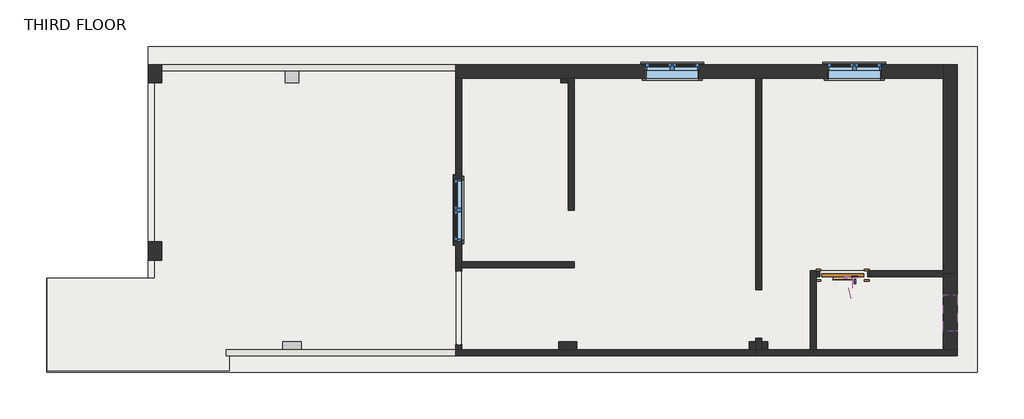
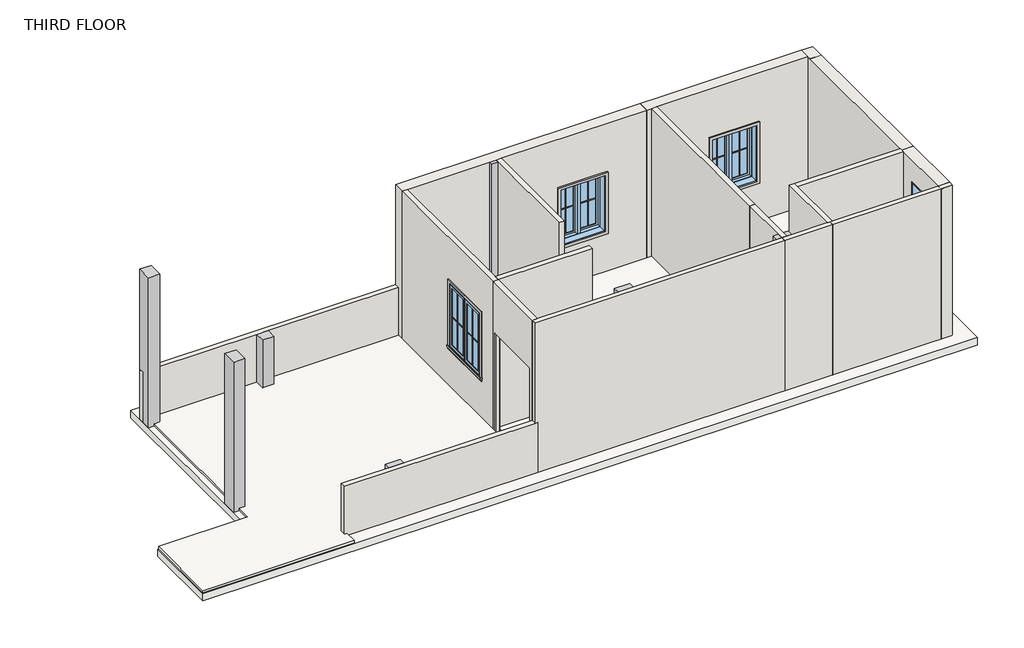
# One storey, incomplete: 16 walls, 13 proxies, 10 columns, 4 slabs, 4 windows, 1 door.
"""IFC4 building model written with IfcOpenShell, lengths in millimetres."""

from ifc_helpers import new_model, si_unit, frame, origin, place, context, project, spatial, polyline, outline, extrude, faceted_brep, transform, mapped, element, save
from components import bel_door_closer_bel_door_closer_f210e2f3, muntin_pattern_2x2_muntin_pattern_2x2_1acec82f, muntin_pattern_2x2_muntin_pattern_2x2_43d02eee, muntin_pattern_2x2_muntin_pattern_2x2_88bf7f41, muntin_pattern_2x2_muntin_pattern_2x2_3dfd0a47, trim_window_exterior_flat_with_sill_e4b28ec3, trim_window_exterior_flat_with_sill_4930676f, trim_window_interior_flat_picture_frame_39ff4276, trim_window_interior_flat_picture_frame_dd064338, apartment_toilet_door_15897_d3_toilet_d7560075, window_80340324, window_6ac8034a, window_casement_double_w1_d341e8ac

model = new_model("IFC4")

# Units and contexts
model_context = context("Model", 3, world=origin())
ifc_project = project(units=[si_unit("LENGTHUNIT", "METRE", prefix="MILLI")], contexts=[model_context])

# Site, building, storey
site = spatial("IfcSite", under=ifc_project)
building = spatial("IfcBuilding", under=site)
storey = spatial("IfcBuildingStorey", under=building, Name="THIRD FLOOR", Elevation=9601.2)

# Proxies
placement = place(None, origin())
bel_door_closer_bel_door_closer_shape = bel_door_closer_bel_door_closer_f210e2f3(model_context)
element("IfcBuildingElementProxy", 1, Name="BEL-Door Closer : BEL-Door Closer", ObjectType="BEL-Door Closer : BEL-Door Closer", at=placement, inside=storey, context=model_context, shape_type="MappedRepresentation", body=[
    mapped(bel_door_closer_bel_door_closer_shape, transform((6826.3533773, 1546.5642852, 11745.8957985), x_axis=(-1.0, 0.0, 0.0), y_axis=(0.0, 0.0, -1.0), z_axis=(0.0, -1.0, 0.0))),
])
muntin_pattern_2x2_muntin_pattern_2x2_shape = muntin_pattern_2x2_muntin_pattern_2x2_1acec82f(model_context)
element("IfcBuildingElementProxy", 2, Name="Muntin Pattern_2x2 : Muntin Pattern_2x2", ObjectType="Muntin Pattern_2x2 : Muntin Pattern_2x2", at=placement, inside=storey, context=model_context, shape_type="MappedRepresentation", body=[
    mapped(muntin_pattern_2x2_muntin_pattern_2x2_shape, transform((6922.3783773, 5093.0392852, 10585.45), x_axis=(1.0, 0.0, 0.0), y_axis=(0.0, 1.0, 0.0), z_axis=(0.0, 0.0, 1.0))),
])
element("IfcBuildingElementProxy", 3, Name="Muntin Pattern_2x2 : Muntin Pattern_2x2", ObjectType="Muntin Pattern_2x2 : Muntin Pattern_2x2", at=placement, inside=storey, context=model_context, shape_type="MappedRepresentation", body=[
    mapped(muntin_pattern_2x2_muntin_pattern_2x2_shape, transform((3868.0283773, 5093.0392852, 10585.45), x_axis=(1.0, 0.0, 0.0), y_axis=(0.0, 1.0, 0.0), z_axis=(0.0, 0.0, 1.0))),
])
muntin_pattern_2x2_muntin_pattern_2x2_2_shape = muntin_pattern_2x2_muntin_pattern_2x2_43d02eee(model_context)
element("IfcBuildingElementProxy", 4, Name="Muntin Pattern_2x2 : Muntin Pattern_2x2", ObjectType="Muntin Pattern_2x2 : Muntin Pattern_2x2", at=placement, inside=storey, context=model_context, shape_type="MappedRepresentation", body=[
    mapped(muntin_pattern_2x2_muntin_pattern_2x2_2_shape, transform((7376.4033773, 5093.0392852, 10585.45), x_axis=(-1.0, 0.0, 0.0), y_axis=(0.0, -1.0, 0.0), z_axis=(0.0, 0.0, 1.0))),
])
element("IfcBuildingElementProxy", 5, Name="Muntin Pattern_2x2 : Muntin Pattern_2x2", ObjectType="Muntin Pattern_2x2 : Muntin Pattern_2x2", at=placement, inside=storey, context=model_context, shape_type="MappedRepresentation", body=[
    mapped(muntin_pattern_2x2_muntin_pattern_2x2_2_shape, transform((4322.0533773, 5093.0392852, 10585.45), x_axis=(-1.0, 0.0, 0.0), y_axis=(0.0, -1.0, 0.0), z_axis=(0.0, 0.0, 1.0))),
])
muntin_pattern_2x2_muntin_pattern_2x2_3_shape = muntin_pattern_2x2_muntin_pattern_2x2_88bf7f41(model_context)
element("IfcBuildingElementProxy", 6, Name="Muntin Pattern_2x2 : Muntin Pattern_2x2", ObjectType="Muntin Pattern_2x2 : Muntin Pattern_2x2", at=placement, inside=storey, context=model_context, shape_type="MappedRepresentation", body=[
    mapped(muntin_pattern_2x2_muntin_pattern_2x2_3_shape, transform((472.3658773, 2405.4017852, 10585.45), x_axis=(0.0, 1.0, 0.0), y_axis=(-1.0, 0.0, 0.0), z_axis=(0.0, 0.0, 1.0))),
])
muntin_pattern_2x2_muntin_pattern_2x2_4_shape = muntin_pattern_2x2_muntin_pattern_2x2_3dfd0a47(model_context)
element("IfcBuildingElementProxy", 7, Name="Muntin Pattern_2x2 : Muntin Pattern_2x2", ObjectType="Muntin Pattern_2x2 : Muntin Pattern_2x2", at=placement, inside=storey, context=model_context, shape_type="MappedRepresentation", body=[
    mapped(muntin_pattern_2x2_muntin_pattern_2x2_4_shape, transform((472.3658773, 2922.9267852, 10585.45), x_axis=(0.0, -1.0, 0.0), y_axis=(1.0, 0.0, 0.0), z_axis=(0.0, 0.0, 1.0))),
])
trim_window_exterior_flat_with_sill_shape = trim_window_exterior_flat_with_sill_e4b28ec3(model_context)
element("IfcBuildingElementProxy", 8, Name="Trim-Window-Exterior-Flat : with Sill", ObjectType="Trim-Window-Exterior-Flat : with Sill", at=placement, inside=storey, context=model_context, shape_type="MappedRepresentation", body=[
    mapped(trim_window_exterior_flat_with_sill_shape, transform((7149.3908773, 5102.5642852, 11734.8), x_axis=(-1.0, 0.0, 0.0), y_axis=(0.0, 0.0, 1.0), z_axis=(0.0, 1.0, 0.0))),
])
element("IfcBuildingElementProxy", 9, Name="Trim-Window-Exterior-Flat : with Sill", ObjectType="Trim-Window-Exterior-Flat : with Sill", at=placement, inside=storey, context=model_context, shape_type="MappedRepresentation", body=[
    mapped(trim_window_exterior_flat_with_sill_shape, transform((4095.0408773, 5102.5642852, 11734.8), x_axis=(-1.0, 0.0, 0.0), y_axis=(0.0, 0.0, 1.0), z_axis=(0.0, 1.0, 0.0))),
])
trim_window_exterior_flat_with_sill_2_shape = trim_window_exterior_flat_with_sill_4930676f(model_context)
element("IfcBuildingElementProxy", 10, Name="Trim-Window-Exterior-Flat : with Sill", ObjectType="Trim-Window-Exterior-Flat : with Sill", at=placement, inside=storey, context=model_context, shape_type="MappedRepresentation", body=[
    mapped(trim_window_exterior_flat_with_sill_2_shape, transform((462.8408773, 2664.1642852, 11861.8), x_axis=(0.0, -1.0, 0.0), y_axis=(0.0, 0.0, 1.0), z_axis=(-1.0, 0.0, 0.0))),
])
trim_window_interior_flat_picture_frame_shape = trim_window_interior_flat_picture_frame_39ff4276(model_context)
element("IfcBuildingElementProxy", 11, Name="Trim-Window-Interior-Flat : Picture Frame", ObjectType="Trim-Window-Interior-Flat : Picture Frame", at=placement, inside=storey, context=model_context, shape_type="MappedRepresentation", body=[
    mapped(trim_window_interior_flat_picture_frame_shape, transform((7149.3908773, 4873.9642852, 11734.8), x_axis=(1.0, 0.0, 0.0), y_axis=(0.0, 0.0, 1.0), z_axis=(0.0, -1.0, 0.0))),
])
element("IfcBuildingElementProxy", 12, Name="Trim-Window-Interior-Flat : Picture Frame", ObjectType="Trim-Window-Interior-Flat : Picture Frame", at=placement, inside=storey, context=model_context, shape_type="MappedRepresentation", body=[
    mapped(trim_window_interior_flat_picture_frame_shape, transform((4095.0408773, 4873.9642852, 11734.8), x_axis=(1.0, 0.0, 0.0), y_axis=(0.0, 0.0, 1.0), z_axis=(0.0, -1.0, 0.0))),
])
trim_window_interior_flat_picture_frame_2_shape = trim_window_interior_flat_picture_frame_dd064338(model_context)
element("IfcBuildingElementProxy", 13, Name="Trim-Window-Interior-Flat : Picture Frame", ObjectType="Trim-Window-Interior-Flat : Picture Frame", at=placement, inside=storey, context=model_context, shape_type="MappedRepresentation", body=[
    mapped(trim_window_interior_flat_picture_frame_2_shape, transform((564.4408773, 2664.1642852, 11861.8), x_axis=(0.0, 1.0, 0.0), y_axis=(0.0, 0.0, 1.0), z_axis=(1.0, 0.0, 0.0))),
])

# Columns
element("IfcColumn", 14, ObjectType="Rectangular Column : 9\" X 12\"", at=placement, inside=storey, context=model_context, shape_type="Brep", body=[
    faceted_brep([(8641.6408773, 5102.5642852, 9601.2), (8870.2408773, 5102.5642852, 9601.2), (8870.2408773, 4797.7642852, 9601.2), (8641.6408773, 4797.7642852, 9601.2), (8641.6408773, 4873.9642852, 9601.2), (8641.6408773, 5102.5642852, 12801.6), (8870.2408773, 5102.5642852, 12801.6), (8870.2408773, 4797.7642852, 12801.6), (8641.6408773, 4797.7642852, 12801.6), (8641.6408773, 4873.9642852, 12801.6)], [[[0, 1, 2, 3, 4]], [[5, 6, 1, 0]], [[6, 7, 2, 1]], [[7, 8, 3, 2]], [[8, 9, 5, 0, 4, 3]], [[5, 9, 8, 7, 6]]]),
])
element("IfcColumn", 15, ObjectType="Rectangular Column : 9\" X 12\"", at=placement, inside=storey, context=model_context, shape_type="Brep", body=[
    faceted_brep([(5390.4408773, 4873.9642852, 9601.2), (5390.4408773, 5102.5642852, 9601.2), (5695.2408773, 5102.5642852, 9601.2), (5695.2408773, 4873.9642852, 9601.2), (5593.6408773, 4873.9642852, 9601.2), (5492.0408773, 4873.9642852, 9601.2), (5390.4408773, 4873.9642852, 12801.6), (5390.4408773, 5102.5642852, 12801.6), (5695.2408773, 5102.5642852, 12801.6), (5695.2408773, 4873.9642852, 12801.6), (5593.6408773, 4873.9642852, 12801.6), (5492.0408773, 4873.9642852, 12801.6)], [[[0, 1, 2, 3, 4, 5]], [[6, 7, 1, 0]], [[7, 8, 2, 1]], [[8, 9, 3, 2]], [[9, 10, 11, 6, 0, 5, 4, 3]], [[6, 11, 10, 9, 8, 7]]]),
])
element("IfcColumn", 16, ObjectType="Rectangular Column : 9\" X 12\"", at=placement, inside=storey, context=model_context, shape_type="SweptSolid", body=[
    extrude(outline(polyline([(2355.1408773, 4797.7642852), (2228.1408773, 4797.7642852), (2228.1408773, 4873.9642852), (2355.1408773, 4873.9642852), (2355.1408773, 4797.7642852)])), frame((0.0, 0.0, 9601.2), z_axis=(0.0, 0.0, 1.0), x_axis=(1.0, 0.0, 0.0)), (0.0, 0.0, 1.0), 3200.4),
])
element("IfcColumn", 17, ObjectType="Rectangular Column : 9\" X 12\"", at=placement, inside=storey, context=model_context, shape_type="SweptSolid", body=[
    extrude(outline(polyline([(-2166.0591227, 4797.7642852), (-2394.6591227, 4797.7642852), (-2394.6591227, 5000.9642852), (-2166.0591227, 5000.9642852), (-2166.0591227, 4797.7642852)])), frame((0.0, 0.0, 9601.2), z_axis=(0.0, 0.0, 1.0), x_axis=(1.0, 0.0, 0.0)), (0.0, 0.0, 1.0), 1066.8),
])
element("IfcColumn", 18, ObjectType="Rectangular Column : 9\" X 12\"", at=placement, inside=storey, context=model_context, shape_type="SweptSolid", body=[
    extrude(outline(polyline([(4797.7642852, 9601.2), (4797.7642852, 12801.6), (5102.5642852, 12801.6), (5102.5642852, 10668.0), (5000.9642852, 10668.0), (5000.9642852, 9601.2), (4797.7642852, 9601.2)])), frame((-4693.3591227, 0.0, 0.0), z_axis=(1.0, 0.0, 0.0), x_axis=(0.0, 1.0, 0.0)), (0.0, 0.0, 1.0), 228.6),
])
element("IfcColumn", 19, ObjectType="Rectangular Column : 9\" X 12\"", at=placement, inside=storey, context=model_context, shape_type="SweptSolid", body=[
    extrude(outline(polyline([(8870.2408773, 225.7642852), (8641.6408773, 225.7642852), (8641.6408773, 327.3642852), (8870.2408773, 327.3642852), (8870.2408773, 225.7642852)])), frame((0.0, 0.0, 9601.2), z_axis=(0.0, 0.0, 1.0), x_axis=(1.0, 0.0, 0.0)), (0.0, 0.0, 1.0), 3200.4),
])
element("IfcColumn", 20, ObjectType="Rectangular Column : 9\" X 12\"", at=placement, inside=storey, context=model_context, shape_type="SweptSolid", body=[
    extrude(outline(polyline([(5390.4408773, 454.3642852), (5492.0408773, 454.3642852), (5492.0408773, 327.3642852), (5390.4408773, 327.3642852), (5390.4408773, 454.3642852)])), frame((0.0, 0.0, 9601.2), z_axis=(0.0, 0.0, 1.0), x_axis=(1.0, 0.0, 0.0)), (0.0, 0.0, 1.0), 3200.4),
    extrude(outline(polyline([(5593.6408773, 454.3642852), (5695.2408773, 454.3642852), (5695.2408773, 327.3642852), (5593.6408773, 327.3642852), (5593.6408773, 454.3642852)])), frame((0.0, 0.0, 9601.2), z_axis=(0.0, 0.0, 1.0), x_axis=(1.0, 0.0, 0.0)), (0.0, 0.0, 1.0), 3200.4),
])
element("IfcColumn", 21, ObjectType="Rectangular Column : 9\" X 12\"", at=placement, inside=storey, context=model_context, shape_type="SweptSolid", body=[
    extrude(outline(polyline([(2190.0408773, 454.3642852), (2494.8408773, 454.3642852), (2494.8408773, 327.3642852), (2190.0408773, 327.3642852), (2190.0408773, 454.3642852)])), frame((0.0, 0.0, 9601.2), z_axis=(0.0, 0.0, 1.0), x_axis=(1.0, 0.0, 0.0)), (0.0, 0.0, 1.0), 3200.4),
])
element("IfcColumn", 22, ObjectType="Rectangular Column : 9\" X 12\"", at=placement, inside=storey, context=model_context, shape_type="SweptSolid", body=[
    extrude(outline(polyline([(-2432.7591227, 454.3642852), (-2127.9591227, 454.3642852), (-2127.9591227, 327.3642852), (-2432.7591227, 327.3642852), (-2432.7591227, 454.3642852)])), frame((0.0, 0.0, 9601.2), z_axis=(0.0, 0.0, 1.0), x_axis=(1.0, 0.0, 0.0)), (0.0, 0.0, 1.0), 1066.8),
])
element("IfcColumn", 23, ObjectType="Rectangular Column : 9\" X 12\"", at=placement, inside=storey, context=model_context, shape_type="SweptSolid", body=[
    extrude(outline(polyline([(-4693.3591227, 2130.7642852), (-4464.7591227, 2130.7642852), (-4464.7591227, 1825.9642852), (-4693.3591227, 1825.9642852), (-4693.3591227, 2130.7642852)])), frame((0.0, 0.0, 9601.2), z_axis=(0.0, 0.0, 1.0), x_axis=(1.0, 0.0, 0.0)), (0.0, 0.0, 1.0), 3200.4),
])

# Door
apartment_toilet_door_15897_d3_toilet_shape = apartment_toilet_door_15897_d3_toilet_d7560075(model_context)
element("IfcDoor", 24, ObjectType="Apartment_Toilet_Door_15897 : D3 TOILET", at=placement, inside=storey, context=model_context, shape_type="MappedRepresentation", body=[
    mapped(apartment_toilet_door_15897_d3_toilet_shape, transform((6952.5408773, 1597.3642852, 9601.2), x_axis=(-1.0, 0.0, 0.0), y_axis=(0.0, -1.0, 0.0), z_axis=(0.0, 0.0, 1.0))),
])

# Slabs
element("IfcSlab", 25, ObjectType="6\" SLAB", at=placement, inside=storey, context=model_context, shape_type="SweptSolid", body=[
    extrude(outline(polyline([(9213.1408773, 5407.3642852), (9213.1408773, 113.4304234), (9213.1408773, -53.6357148), (-6395.1591227, -53.6357148), (-6395.1591227, 1521.1642852), (-4693.3591227, 1521.1642852), (-4693.3591227, 5407.3642852), (9213.1408773, 5407.3642852)])), frame((0.0, 0.0, 9448.8), z_axis=(0.0, 0.0, 1.0), x_axis=(1.0, 0.0, 0.0)), (0.0, 0.0, 1.0), 152.4),
])
element("IfcSlab", 26, ObjectType="FLOORING", at=placement, inside=storey, context=model_context, shape_type="SweptSolid", body=[
    extrude(outline(polyline([(5492.0408773, 327.3642852), (564.4408773, 327.3642852), (564.4408773, 1698.9642852), (2456.7408773, 1698.9642852), (2456.7408773, 1800.5642852), (564.4408773, 1800.5642852), (564.4408773, 4873.9642852), (2228.1408773, 4873.9642852), (2228.1408773, 4797.7642852), (2355.1408773, 4797.7642852), (2355.1408773, 2664.1642852), (2456.7408773, 2664.1642852), (2456.7408773, 4873.9642852), (5492.0408773, 4873.9642852), (5492.0408773, 1330.6642852), (5593.6408773, 1330.6642852), (5593.6408773, 4873.9642852), (8641.6408773, 4873.9642852), (8641.6408773, 1648.1642852), (6406.4408773, 1648.1642852), (6406.4408773, 327.3642852), (5593.6408773, 327.3642852), (5593.6408773, 517.8642852), (5492.0408773, 517.8642852), (5492.0408773, 327.3642852)])), frame((0.0, 0.0, 9601.2), z_axis=(0.0, 0.0, 1.0), x_axis=(1.0, 0.0, 0.0)), (0.0, 0.0, 1.0), 50.8),
])
element("IfcSlab", 27, ObjectType="FLOORING OPEN AREA", at=placement, inside=storey, context=model_context, shape_type="SweptSolid", body=[
    extrude(outline(polyline([(462.8408773, 5000.9642852), (462.8408773, 327.3642852), (-2127.9591227, 327.3642852), (-2127.9591227, 454.3642852), (-2432.7591227, 454.3642852), (-2432.7591227, 327.3642852), (-3385.2591227, 327.3642852), (-3385.2591227, 225.7642852), (-3334.4591227, 225.7642852), (-3334.4591227, -28.2357148), (-6382.4591227, -28.2357148), (-6382.4591227, 1521.1642852), (-4579.0591227, 1521.1642852), (-4579.0591227, 4797.7642852), (-4464.7591227, 4797.7642852), (-4464.7591227, 5000.9642852), (462.8408773, 5000.9642852)])), frame((0.0, 0.0, 9601.2), z_axis=(0.0, 0.0, 1.0), x_axis=(1.0, 0.0, 0.0)), (0.0, 0.0, 1.0), 50.8),
])
element("IfcSlab", 28, ObjectType="FLOORING TOILET", at=placement, inside=storey, context=model_context, shape_type="SweptSolid", body=[
    extrude(outline(polyline([(6508.0408773, 327.3642852), (6508.0408773, 1546.5642852), (6571.5408773, 1546.5642852), (6571.5408773, 1648.1642852), (7371.5408773, 1648.1642852), (7371.5408773, 1546.5642852), (8641.6408773, 1546.5642852), (8641.6408773, 327.3642852), (6508.0408773, 327.3642852)])), frame((0.0, 0.0, 9601.2), z_axis=(0.0, 0.0, 1.0), x_axis=(1.0, 0.0, 0.0)), (0.0, 0.0, 1.0), 50.8),
])

# Walls
element("IfcWall", 29, ObjectType="4\" WALL", at=placement, inside=storey, context=model_context, shape_type="Brep", body=[
    faceted_brep([(8870.2408773, 327.3642852, 9601.2), (8641.6408773, 327.3642852, 9601.2), (6508.0408773, 327.3642852, 9601.2), (6457.2408773, 327.3642852, 9601.2), (6457.2408773, 327.3642852, 12801.6), (6508.0408773, 327.3642852, 12801.6), (8641.6408773, 327.3642852, 12801.6), (8870.2408773, 327.3642852, 12801.6), (8870.2408773, 225.7642852, 9601.2), (8870.2408773, 225.7642852, 12801.6), (6457.2408773, 225.7642852, 12801.6), (6457.2408773, 225.7642852, 9601.2)], [[[0, 1, 2, 3, 4, 5, 6, 7]], [[8, 9, 10, 11]], [[3, 2, 1, 0, 8, 11]], [[4, 3, 11, 10]], [[7, 6, 5, 4, 10, 9]], [[0, 7, 9, 8]]]),
])
element("IfcWall", 30, ObjectType="4\" WALL", at=placement, inside=storey, context=model_context, shape_type="Brep", body=[
    faceted_brep([(5593.6408773, 1444.9642852, 9601.2), (5593.6408773, 1444.9642852, 12801.6), (5593.6408773, 454.3642852, 12801.6), (5593.6408773, 327.3642852, 12801.6), (5593.6408773, 327.3642852, 9601.2), (5593.6408773, 454.3642852, 9601.2), (5593.6408773, 517.8642852, 9601.2), (5593.6408773, 517.8642852, 11734.8), (5593.6408773, 1330.6642852, 11734.8), (5593.6408773, 1330.6642852, 9601.2), (5492.0408773, 1444.9642852, 12801.6), (5492.0408773, 1444.9642852, 9601.2), (5492.0408773, 1330.6642852, 9601.2), (5492.0408773, 1330.6642852, 11734.8), (5492.0408773, 517.8642852, 11734.8), (5492.0408773, 517.8642852, 9601.2), (5492.0408773, 454.3642852, 9601.2), (5492.0408773, 327.3642852, 9601.2), (5492.0408773, 327.3642852, 12801.6), (5492.0408773, 454.3642852, 12801.6)], [[[0, 1, 2, 3, 4, 5, 6, 7, 8, 9]], [[10, 11, 12, 13, 14, 15, 16, 17, 18, 19]], [[4, 17, 16, 15, 6, 5]], [[11, 0, 9, 12]], [[1, 0, 11, 10]], [[3, 2, 1, 10, 19, 18]], [[4, 3, 18, 17]], [[14, 7, 6, 15]], [[7, 14, 13, 8]], [[8, 13, 12, 9]]]),
])
element("IfcWall", 31, ObjectType="4\" WALL", at=placement, inside=storey, context=model_context, shape_type="Brep", body=[
    faceted_brep([(6508.0408773, 327.3642852, 9601.2), (6508.0408773, 1546.5642852, 9601.2), (6508.0408773, 1648.1642852, 9601.2), (6508.0408773, 1648.1642852, 12801.6), (6508.0408773, 1546.5642852, 12801.6), (6508.0408773, 327.3642852, 12801.6), (6406.4408773, 327.3642852, 9601.2), (6406.4408773, 327.3642852, 12801.6), (6406.4408773, 1648.1642852, 12801.6), (6406.4408773, 1648.1642852, 9601.2), (6457.2408773, 327.3642852, 9601.2), (6457.2408773, 327.3642852, 12801.6)], [[[0, 1, 2, 3, 4, 5]], [[6, 7, 8, 9]], [[2, 1, 0, 10, 6, 9]], [[5, 4, 3, 8, 7, 11]], [[0, 5, 11, 7, 6, 10]], [[3, 2, 9, 8]]]),
])
element("IfcWall", 32, ObjectType="4\" WALL", at=placement, inside=storey, context=model_context, shape_type="Brep", body=[
    faceted_brep([(6508.0408773, 1546.5642852, 9601.2), (6571.5408773, 1546.5642852, 9601.2), (6571.5408773, 1546.5642852, 11734.8), (7371.5408773, 1546.5642852, 11734.8), (7371.5408773, 1546.5642852, 9601.2), (8641.6408773, 1546.5642852, 9601.2), (8641.6408773, 1546.5642852, 12801.6), (6508.0408773, 1546.5642852, 12801.6), (6571.5408773, 1648.1642852, 11734.8), (6571.5408773, 1648.1642852, 9601.2), (6508.0408773, 1648.1642852, 9601.2), (6508.0408773, 1648.1642852, 12801.6), (8641.6408773, 1648.1642852, 12801.6), (8641.6408773, 1648.1642852, 9601.2), (7371.5408773, 1648.1642852, 9601.2), (7371.5408773, 1648.1642852, 11734.8), (8641.6408773, 1597.3642852, 9601.2), (8641.6408773, 1597.3642852, 12801.6)], [[[0, 1, 2, 3, 4, 5, 6, 7]], [[8, 9, 10, 11, 12, 13, 14, 15]], [[14, 13, 16, 5, 4]], [[10, 9, 1, 0]], [[7, 6, 17, 12, 11]], [[0, 7, 11, 10]], [[6, 5, 16, 13, 12, 17]], [[2, 1, 9, 8]], [[3, 2, 8, 15]], [[4, 3, 15, 14]]]),
])
element("IfcWall", 33, ObjectType="4\" WALL", at=placement, inside=storey, context=model_context, shape_type="SweptSolid", body=[
    extrude(outline(polyline([(5593.6408773, 4873.9642852), (5593.6408773, 1444.9642852), (5492.0408773, 1444.9642852), (5492.0408773, 4873.9642852), (5593.6408773, 4873.9642852)])), frame((0.0, 0.0, 9601.2), z_axis=(0.0, 0.0, 1.0), x_axis=(1.0, 0.0, 0.0)), (0.0, 0.0, 1.0), 3200.4),
])
element("IfcWall", 34, ObjectType="4\" WALL", at=placement, inside=storey, context=model_context, shape_type="Brep", body=[
    faceted_brep([(6457.2408773, 327.3642852, 9601.2), (6406.4408773, 327.3642852, 9601.2), (5695.2408773, 327.3642852, 9601.2), (5593.6408773, 327.3642852, 9601.2), (5492.0408773, 327.3642852, 9601.2), (5492.0408773, 327.3642852, 12801.6), (5593.6408773, 327.3642852, 12801.6), (5695.2408773, 327.3642852, 12801.6), (6406.4408773, 327.3642852, 12801.6), (6457.2408773, 327.3642852, 12801.6), (6457.2408773, 225.7642852, 9601.2), (6457.2408773, 225.7642852, 12801.6), (5492.0408773, 225.7642852, 12801.6), (5492.0408773, 225.7642852, 9601.2)], [[[0, 1, 2, 3, 4, 5, 6, 7, 8, 9]], [[10, 11, 12, 13]], [[4, 3, 2, 1, 0, 10, 13]], [[9, 8, 7, 6, 5, 12, 11]], [[0, 9, 11, 10]], [[5, 4, 13, 12]]]),
])
element("IfcWall", 35, ObjectType="4\" WALL", at=placement, inside=storey, context=model_context, shape_type="Brep", body=[
    faceted_brep([(2456.7408773, 2664.1642852, 9601.2), (2456.7408773, 4873.9642852, 9601.2), (2456.7408773, 4873.9642852, 12801.6), (2456.7408773, 2664.1642852, 12801.6), (2355.1408773, 2664.1642852, 9601.2), (2355.1408773, 2664.1642852, 12801.6), (2355.1408773, 4797.7642852, 12801.6), (2355.1408773, 4873.9642852, 12801.6), (2355.1408773, 4873.9642852, 9601.2), (2355.1408773, 4797.7642852, 9601.2)], [[[0, 1, 2, 3]], [[4, 5, 6, 7, 8, 9]], [[1, 0, 4, 9, 8]], [[3, 2, 7, 6, 5]], [[0, 3, 5, 4]], [[2, 1, 8, 7]]]),
])
element("IfcWall", 36, ObjectType="4\" WALL", at=placement, inside=storey, context=model_context, shape_type="Brep", body=[
    faceted_brep([(462.8408773, 4873.9642852, 12801.6), (462.8408773, 4873.9642852, 9601.2), (462.8408773, 1698.9642852, 9601.2), (462.8408773, 1698.9642852, 12801.6), (462.8408773, 3184.8642852, 11861.8), (462.8408773, 2143.4642852, 11861.8), (462.8408773, 2143.4642852, 10515.6), (462.8408773, 3184.8642852, 10515.6), (564.4408773, 4873.9642852, 9601.2), (564.4408773, 4873.9642852, 12801.6), (564.4408773, 1800.5642852, 12801.6), (564.4408773, 1698.9642852, 12801.6), (564.4408773, 1698.9642852, 9601.2), (564.4408773, 1800.5642852, 9601.2), (564.4408773, 3184.8642852, 11861.8), (564.4408773, 3184.8642852, 10515.6), (564.4408773, 2143.4642852, 10515.6), (564.4408773, 2143.4642852, 11861.8)], [[[0, 1, 2, 3], [4, 5, 6, 7]], [[8, 9, 10, 11, 12, 13], [14, 15, 16, 17]], [[2, 1, 8, 13, 12]], [[0, 3, 11, 10, 9]], [[3, 2, 12, 11]], [[15, 14, 4, 7]], [[16, 15, 7, 6]], [[17, 16, 6, 5]], [[14, 17, 5, 4]], [[0, 9, 8, 1]]]),
])
element("IfcWall", 37, ObjectType="4\" WALL", at=placement, inside=storey, context=model_context, shape_type="SweptSolid", body=[
    extrude(outline(polyline([(564.4408773, 1800.5642852), (2456.7408773, 1800.5642852), (2456.7408773, 1698.9642852), (564.4408773, 1698.9642852), (564.4408773, 1800.5642852)])), frame((0.0, 0.0, 9601.2), z_axis=(0.0, 0.0, 1.0), x_axis=(1.0, 0.0, 0.0)), (0.0, 0.0, 1.0), 3200.4),
])
element("IfcWall", 38, ObjectType="4\" WALL", at=placement, inside=storey, context=model_context, shape_type="Brep", body=[
    faceted_brep([(5492.0408773, 327.3642852, 9601.2), (5390.4408773, 327.3642852, 9601.2), (2494.8408773, 327.3642852, 9601.2), (2190.0408773, 327.3642852, 9601.2), (564.4408773, 327.3642852, 9601.2), (513.6408773, 327.3642852, 9601.2), (513.6408773, 327.3642852, 10668.0), (462.8408773, 327.3642852, 10668.0), (462.8408773, 327.3642852, 12801.6), (564.4408773, 327.3642852, 12801.6), (2190.0408773, 327.3642852, 12801.6), (2494.8408773, 327.3642852, 12801.6), (5390.4408773, 327.3642852, 12801.6), (5492.0408773, 327.3642852, 12801.6), (5492.0408773, 225.7642852, 9601.2), (5492.0408773, 225.7642852, 12801.6), (462.8408773, 225.7642852, 12801.6), (462.8408773, 225.7642852, 10668.0), (513.6408773, 225.7642852, 10668.0), (513.6408773, 225.7642852, 9601.2)], [[[0, 1, 2, 3, 4, 5, 6, 7, 8, 9, 10, 11, 12, 13]], [[14, 15, 16, 17, 18, 19]], [[5, 4, 3, 2, 1, 0, 14, 19]], [[13, 12, 11, 10, 9, 8, 16, 15]], [[6, 5, 19, 18]], [[17, 7, 6, 18]], [[8, 7, 17, 16]], [[0, 13, 15, 14]]]),
])
element("IfcWall", 39, ObjectType="4\" WALL", at=placement, inside=storey, context=model_context, shape_type="Brep", body=[
    faceted_brep([(564.4408773, 1698.9642852, 12801.6), (564.4408773, 327.3642852, 12801.6), (564.4408773, 327.3642852, 9601.2), (564.4408773, 416.2642852, 9601.2), (564.4408773, 416.2642852, 11734.8), (564.4408773, 1635.4642852, 11734.8), (564.4408773, 1635.4642852, 9601.2), (564.4408773, 1698.9642852, 9601.2), (462.8408773, 327.3642852, 12801.6), (462.8408773, 1698.9642852, 12801.6), (462.8408773, 1698.9642852, 9601.2), (462.8408773, 1635.4642852, 9601.2), (462.8408773, 1635.4642852, 11734.8), (462.8408773, 416.2642852, 11734.8), (462.8408773, 416.2642852, 9601.2), (462.8408773, 327.3642852, 9601.2), (462.8408773, 327.3642852, 10668.0), (559.8408773, 1635.4642852, 9601.2), (559.8408773, 1650.4642852, 9601.2), (482.8408773, 1650.4642852, 9601.2), (482.8408773, 1635.4642852, 9601.2), (513.6408773, 327.3642852, 9601.2), (482.8408773, 416.2642852, 9601.2), (482.8408773, 401.2642852, 9601.2), (559.8408773, 401.2642852, 9601.2), (559.8408773, 416.2642852, 9601.2), (482.8408773, 1635.4642852, 11734.8), (482.8408773, 416.2642852, 11734.8), (482.8408773, 1650.4642852, 11749.8), (482.8408773, 401.2642852, 11749.8), (559.8408773, 1650.4642852, 11749.8), (559.8408773, 1635.4642852, 11734.8), (559.8408773, 416.2642852, 11734.8), (559.8408773, 401.2642852, 11749.8)], [[[0, 1, 2, 3, 4, 5, 6, 7]], [[8, 9, 10, 11, 12, 13, 14, 15, 16]], [[10, 7, 6, 17, 18, 19, 20, 11]], [[2, 21, 15, 14, 22, 23, 24, 25, 3]], [[1, 0, 9, 8]], [[0, 7, 10, 9]], [[20, 26, 12, 11]], [[27, 22, 14, 13]], [[26, 27, 13, 12]], [[26, 20, 19, 28, 29, 23, 22, 27]], [[28, 19, 18, 30]], [[30, 18, 17, 31, 32, 25, 24, 33]], [[29, 28, 30, 33]], [[23, 29, 33, 24]], [[31, 17, 6, 5]], [[25, 32, 4, 3]], [[32, 31, 5, 4]], [[1, 8, 16, 15, 21, 2]]]),
])
element("IfcWall", 40, ObjectType="4\" WALL", at=placement, inside=storey, context=model_context, shape_type="Brep", body=[
    faceted_brep([(462.8408773, 5102.5642852, 9601.2), (-4693.3591227, 5102.5642852, 9601.2), (-4693.3591227, 5102.5642852, 10668.0), (-4464.7591227, 5102.5642852, 10668.0), (462.8408773, 5102.5642852, 10668.0), (462.8408773, 5000.9642852, 9601.2), (462.8408773, 5000.9642852, 10668.0), (-2166.0591227, 5000.9642852, 10668.0), (-2394.6591227, 5000.9642852, 10668.0), (-4464.7591227, 5000.9642852, 10668.0), (-4693.3591227, 5000.9642852, 10668.0), (-4693.3591227, 5000.9642852, 9601.2), (-4464.7591227, 5000.9642852, 9601.2), (-2394.6591227, 5000.9642852, 9601.2), (-2166.0591227, 5000.9642852, 9601.2)], [[[0, 1, 2, 3, 4]], [[5, 6, 7, 8, 9, 10, 11, 12, 13, 14]], [[1, 0, 5, 14, 13, 12, 11]], [[2, 1, 11, 10]], [[4, 3, 2, 10, 9, 8, 7, 6]], [[0, 4, 6, 5]]]),
])
element("IfcWall", 41, ObjectType="4\" WALL", at=placement, inside=storey, context=model_context, shape_type="Brep", body=[
    faceted_brep([(513.6408773, 327.3642852, 9601.2), (462.8408773, 327.3642852, 9601.2), (-2127.9591227, 327.3642852, 9601.2), (-2432.7591227, 327.3642852, 9601.2), (-3385.2591227, 327.3642852, 9601.2), (-3385.2591227, 327.3642852, 10668.0), (-2432.7591227, 327.3642852, 10668.0), (-2127.9591227, 327.3642852, 10668.0), (462.8408773, 327.3642852, 10668.0), (513.6408773, 327.3642852, 10668.0), (513.6408773, 225.7642852, 9601.2), (513.6408773, 225.7642852, 10668.0), (462.8408773, 225.7642852, 10668.0), (-3385.2591227, 225.7642852, 10668.0), (-3385.2591227, 225.7642852, 9601.2)], [[[0, 1, 2, 3, 4, 5, 6, 7, 8, 9]], [[10, 11, 12, 13, 14]], [[4, 3, 2, 1, 0, 10, 14]], [[5, 4, 14, 13]], [[9, 8, 7, 6, 5, 13, 12, 11]], [[0, 9, 11, 10]]]),
])
element("IfcWall", 42, ObjectType="9\" WALL", at=placement, inside=storey, context=model_context, shape_type="Brep", body=[
    faceted_brep([(8641.6408773, 5102.5642852, 9601.2), (462.8408773, 5102.5642852, 9601.2), (462.8408773, 5102.5642852, 10668.0), (462.8408773, 5102.5642852, 12801.6), (8641.6408773, 5102.5642852, 12801.6), (7606.5908773, 5102.5642852, 11734.8), (6692.1908773, 5102.5642852, 11734.8), (6692.1908773, 5102.5642852, 10515.6), (7606.5908773, 5102.5642852, 10515.6), (4552.2408773, 5102.5642852, 11734.8), (3637.8408773, 5102.5642852, 11734.8), (3637.8408773, 5102.5642852, 10515.6), (4552.2408773, 5102.5642852, 10515.6), (8641.6408773, 4873.9642852, 9601.2), (8641.6408773, 4873.9642852, 12801.6), (5593.6408773, 4873.9642852, 12801.6), (5492.0408773, 4873.9642852, 12801.6), (2456.7408773, 4873.9642852, 12801.6), (2355.1408773, 4873.9642852, 12801.6), (2228.1408773, 4873.9642852, 12801.6), (564.4408773, 4873.9642852, 12801.6), (462.8408773, 4873.9642852, 12801.6), (462.8408773, 4873.9642852, 9601.2), (564.4408773, 4873.9642852, 9601.2), (2228.1408773, 4873.9642852, 9601.2), (2355.1408773, 4873.9642852, 9601.2), (2456.7408773, 4873.9642852, 9601.2), (5492.0408773, 4873.9642852, 9601.2), (5593.6408773, 4873.9642852, 9601.2), (7606.5908773, 4873.9642852, 11734.8), (7606.5908773, 4873.9642852, 10515.6), (6692.1908773, 4873.9642852, 10515.6), (6692.1908773, 4873.9642852, 11734.8), (4552.2408773, 4873.9642852, 11734.8), (4552.2408773, 4873.9642852, 10515.6), (3637.8408773, 4873.9642852, 10515.6), (3637.8408773, 4873.9642852, 11734.8), (462.8408773, 5000.9642852, 9601.2)], [[[0, 1, 2, 3, 4], [5, 6, 7, 8], [9, 10, 11, 12]], [[13, 14, 15, 16, 17, 18, 19, 20, 21, 22, 23, 24, 25, 26, 27, 28], [29, 30, 31, 32], [33, 34, 35, 36]], [[1, 0, 13, 28, 27, 26, 25, 24, 23, 22, 37]], [[4, 3, 21, 20, 19, 18, 17, 16, 15, 14]], [[0, 4, 14, 13]], [[30, 29, 5, 8]], [[31, 30, 8, 7]], [[32, 31, 7, 6]], [[29, 32, 6, 5]], [[33, 36, 10, 9]], [[36, 35, 11, 10]], [[35, 34, 12, 11]], [[34, 33, 9, 12]], [[1, 37, 22, 21, 3, 2]]]),
])
element("IfcWall", 43, ObjectType="9\" WALL", at=placement, inside=storey, context=model_context, shape_type="Brep", body=[
    faceted_brep([(8870.2408773, 327.3642852, 9601.2), (8870.2408773, 1597.3642852, 9601.2), (8870.2408773, 1597.3642852, 12801.6), (8870.2408773, 327.3642852, 12801.6), (8870.2408773, 632.1642852, 12344.4), (8870.2408773, 1241.7642852, 12344.4), (8870.2408773, 1241.7642852, 11734.8), (8870.2408773, 632.1642852, 11734.8), (8641.6408773, 327.3642852, 9601.2), (8641.6408773, 327.3642852, 12801.6), (8641.6408773, 1546.5642852, 12801.6), (8641.6408773, 1597.3642852, 12801.6), (8641.6408773, 1597.3642852, 9601.2), (8641.6408773, 1546.5642852, 9601.2), (8641.6408773, 632.1642852, 12344.4), (8641.6408773, 632.1642852, 11734.8), (8641.6408773, 1241.7642852, 11734.8), (8641.6408773, 1241.7642852, 12344.4)], [[[0, 1, 2, 3], [4, 5, 6, 7]], [[8, 9, 10, 11, 12, 13], [14, 15, 16, 17]], [[1, 0, 8, 13, 12]], [[2, 1, 12, 11]], [[3, 2, 11, 10, 9]], [[0, 3, 9, 8]], [[15, 14, 4, 7]], [[16, 15, 7, 6]], [[17, 16, 6, 5]], [[14, 17, 5, 4]]]),
])
element("IfcWall", 44, ObjectType="9\" WALL", at=placement, inside=storey, context=model_context, shape_type="Brep", body=[
    faceted_brep([(8870.2408773, 1597.3642852, 9601.2), (8870.2408773, 5102.5642852, 9601.2), (8870.2408773, 5102.5642852, 12801.6), (8870.2408773, 1597.3642852, 12801.6), (8641.6408773, 1597.3642852, 9601.2), (8641.6408773, 1597.3642852, 12801.6), (8641.6408773, 1648.1642852, 12801.6), (8641.6408773, 4873.9642852, 12801.6), (8641.6408773, 5102.5642852, 12801.6), (8641.6408773, 5102.5642852, 9601.2), (8641.6408773, 4873.9642852, 9601.2), (8641.6408773, 1648.1642852, 9601.2)], [[[0, 1, 2, 3]], [[4, 5, 6, 7, 8, 9, 10, 11]], [[1, 0, 4, 11, 10, 9]], [[3, 2, 8, 7, 6, 5]], [[0, 3, 5, 4]], [[2, 1, 9, 8]]]),
])

# Windows
window_shape = window_80340324(model_context)
element("IfcWindow", 45, ObjectType="Fixed : 24\" x 24\"", at=placement, inside=storey, context=model_context, shape_type="MappedRepresentation", body=[
    mapped(window_shape, transform((8755.9408773, 898.8642852, 10820.4), x_axis=(0.0, -1.0, 0.0), y_axis=(1.0, 0.0, 0.0), z_axis=(0.0, 0.0, 1.0))),
])
window_2_shape = window_6ac8034a(model_context)
element("IfcWindow", 46, ObjectType="Window-Casement-Double : 41\" x 53\"", at=placement, inside=storey, context=model_context, shape_type="MappedRepresentation", body=[
    mapped(window_2_shape, transform((513.6408773, 2664.1642852, 9601.2), x_axis=(0.0, 1.0, 0.0), y_axis=(-1.0, 0.0, 0.0), z_axis=(0.0, 0.0, 1.0))),
])
window_casement_double_w1_shape = window_casement_double_w1_d341e8ac(model_context)
element("IfcWindow", 47, ObjectType="Window-Casement-Double : w1", at=placement, inside=storey, context=model_context, shape_type="MappedRepresentation", body=[
    mapped(window_casement_double_w1_shape, transform((7149.3908773, 4988.2642852, 9601.2), x_axis=(1.0, 0.0, 0.0), y_axis=(0.0, 1.0, 0.0), z_axis=(0.0, 0.0, 1.0))),
])
element("IfcWindow", 48, ObjectType="Window-Casement-Double : w1", at=placement, inside=storey, context=model_context, shape_type="MappedRepresentation", body=[
    mapped(window_casement_double_w1_shape, transform((4095.0408773, 4988.2642852, 9601.2), x_axis=(1.0, 0.0, 0.0), y_axis=(0.0, 1.0, 0.0), z_axis=(0.0, 0.0, 1.0))),
])

save(model, "model.ifc")

# Revit data of these elements
# Type "BEL-Door Closer : BEL-Door Closer"
#   URL = "http://us.allegion.com/brands/falcon/Pages/default.aspx"
#   Standards Conformance = "as Specified"
#   Specification = ""
#   SpecWizard = ""
#   Send Message = "http://arcat.com/users.pl?action=UserEmail&company=Falcon+Lock&coid=32420&rep=114&fax=&mf="
#   Screw Pack Type = "as Specified"
#   Sales Information = "http://us.allegion.com/irst/Pages/contact_us.aspx"
#   Revision = "R1_02-2014"
#   Product Properties = ""
#   Product Data = "http://www.arcat.com/arcatcos/cos32/arc32420.html"
#   Model = "As Specified"
#   Manufacturer Website = "http://us.allegion.com/brands/falcon/Pages/default.aspx"
#   Manufacturer Phone = ""
#   Manufacturer Fax = ""
#   Manufacturer = "Falcon"
#   Keynote = "08710"
#   Installation-Fabrication = ""
#   Installation Phase = ""
#   Green Building-LEED = ""
#   Function Type = "as Specified"
#   Door Type = "as Specified"
#   Description = "Falcon Closer as Specified"
#   Copyright = "©Arcat Inc."
#   Construction Details = ""
#   Assembly Code = "C1020410"
#   originlocate [instance default] = 0' - 0"
#   locatearm [instance default] = 0' - 0 1/2"
#   Unit Width = 0' - 7.87402"
#   Unit Height = 0' - 3.14961"
#   Unit Depth = 0' - 1.1811"
#   Plate Thickness = 0' - 0 1/4"
#   Offset from Edge of Frame_Closer Arm [instance default] = 0' - 7"
#   Offset from Edge of Door_Closer Case [instance default] = 0' - 3 15/16"
#   Offset for Plate [instance default] = 0' - 0"
#   Reveal Between Door and Frame_Right [instance default] = 0' - 0 1/4"
#   Reveal Between Door and Frame_Left [instance default] = 0' - 0 1/4"
#   Door Leaf Width [instance default] = 3' - 0"
#   Door Leaf Top Reveal [instance default] = 0' - 0 1/4"
#   Door Leaf Thickness [instance default] = 0' - 0"
#   Closer Case Side Offset = 0' - 3 15/16"
#   Closer Arm Offset = 0' - 7"
#   Arm Width = 1' - 2"
#   Arm Height = 0' - 1 5/8"
#   Arm Extension [instance default] = 0' - 0"
#   Arm Depth = 1' - 2"
#   ActualArm Height [instance default] = 0' - 1 7/8"
#   ActualArm Depth [instance default] = 1' - 2"
#   Warranty Duration (Years) = 0
#   RH Hinge [instance default] = no
#   Maintenance Schedule (Months) = 0
#   LH Hinge [instance default] = yes
#   Include Mounting Plate [instance default] = no
#   Expected Lifespan (Years) = 0
#   Closer on Door Surface = yes
#   Closer on Door Frame = no
#   Arm Below Closer = no
#   Arm Above Closer = yes
#   Cover Material [instance default] = Metal - IR - Satin Chrome
#   Arm Type = element 418778
#   Arm Material [instance default] = Metal - IR - Satin Chrome
#   Default Elevation = 0
# Type "Muntin Pattern_2x2 : Muntin Pattern_2x2"
#   Width [instance default] = 4' - 0"
#   Thickness = 0' - 0 1/2"
#   Height [instance default] = 4' - 0"
#   Distance = 0' - 0 3/4"
#   Interior Material [instance default] = none
#   Exterior Material [instance default] = none
#   Default Elevation = 0
# Type "Trim-Window-Exterior-Flat : with Sill"
#   Trim Width = 0' - 2 1/4"
#   Trim Thickness_Picture Frame = 0' - 1 1/4"
#   Trim Thickness_with Sill = 0' - 0 3/4"
#   Sill Thickness = 0' - 1 1/4"
#   Opening Width [instance default] = 2' - 0"
#   Opening Height [instance default] = 3' - 0"
#   Default Elevation = 4' - 0"
#   Sill = yes
#   Picture Frame = no
#   Trim Material [instance default] = none
# Type "Trim-Window-Interior-Flat : Picture Frame"
#   Trim Thickness_Picture Frame = 0' - 1 1/4"
#   Trim Width = 0' - 2 1/4"
#   Trim Thickness_with Sill = 0' - 0 3/4"
#   Sill Thickness = 0' - 1 1/4"
#   Opening Width [instance default] = 2' - 0"
#   Opening Height [instance default] = 3' - 0"
#   Default Elevation = 4' - 0"
#   Sill = no
#   Picture Frame = yes
#   Trim Material [instance default] = none
# Type "Rectangular Column : 9\" X 12\""
#   Assembly Code = "B1010200"
#   Depth = 0' - 9"
#   Offset Base = 0' - 0"
#   Offset Top = 0' - 0"
#   Width = 1' - 0"
#   Material = none
# Type "Apartment_Toilet_Door_15897 : D3 TOILET"
#   Type Mark = "15"
#   Panel Type = ""
#   Location [instance default] = ""
#   Door Type = "Semi Solid Flushed Wooden Door Laminated on Boths Sides- Bathroom / Laundry"
#   Construction Type Id = "DOOR"
#   Analytic Construction = "Wooden"
#   Threshold Depth = 0' - 1.1811"
#   Thickness = 0' - 2.12598"
#   Thermal Resistance (R) = 2.58758 (h·ft²·°F)/BTU
#   Heat Transfer Coefficient (U) = 0.386456 BTU/(h·ft²·°F)
#   Height = 7' - 0"
#   Trim Projection Ext = 0' - 0.98425"
#   Trim Projection Int = 0' - 0.98425"
#   Width = 2' - 6"
#   Define Thermal Properties by = 1
#   Threshold Material = BEL-Threshold material-Marble
#   Visual Light Transmittance = 0
#   Solar Heat Gain Coefficient = 0
#   Function = (empty or 0)
#   Wall Closure = (empty or 0)
# Type "6\" SLAB"
#   Assembly Code = "B1010"
#   Function = 0
#   Layers, outside or top first: 0' - 6" "Concrete, Lightweight" (function 1)
# Type "FLOORING"
#   Assembly Code = "B1010"
#   Function = 0
#   Layers, outside or top first: 0' - 2" "FLOORING" (function 1)
# Type "FLOORING OPEN AREA"
#   Assembly Code = "B1010"
#   Function = 0
#   Layers, outside or top first: 0' - 2" "OPEN AREA TILE" (function 1)
# Type "FLOORING TOILET"
#   Assembly Code = "B1010"
#   Function = 0
#   Layers, outside or top first: 0' - 2" "toilet wash room" (function 1)
# Type "4\" WALL"
#   Assembly Code = "B2010"
#   Layers, outside or top first: 0' - 4" "Brick, Common" (function 1)
# Type "9\" WALL"
#   Assembly Code = "B2010"
#   Layers, outside or top first: 0' - 9" "Brick, Common" (function 1)
# Type "Fixed : 24\" x 24\""
#   Type Mark = "4"
#   Construction Type Id = "GSP4R"
#   Assembly Code = "B2020100"
#   Analytic Construction = "1/8 in Pilkington single glazing"
#   Visual Light Transmittance = 0.9
#   Solar Heat Gain Coefficient = 0.78
#   Heat Transfer Coefficient (U) = 0.6496 BTU/(h·ft²·°F)
#   Height = 2' - 0"
#   Default Sill Height = 3' - 0"
#   Width = 2' - 0"
#   Window Inset = 0' - 0 3/4"
#   Define Thermal Properties by = 1
#   Define Thermal Properties by = 1
#   Glass Pane Material = Glass
#   Sash Material = Sash
#   Wall Closure = (empty or 0)
# Type "Window-Casement-Double : 41\" x 53\""
#   Type Mark = "15"
#   Fire Rating = "0.5h"
#   Assembly Code = "B2020100"
#   Analytic Construction = "Double glazing - domestic"
#   Frame Extension [instance default] = 0' - 0 1/4"
#   Window Inset [instance default] = 0' - 0"
#   Wall Thickness [instance default] = 0' - 6"
#   Interior Wall Closure [instance default] = 0' - 2 1/4"
#   Half Width = 1' - 8 1/2"
#   Visual Light Transmittance = 0.81
#   Thermal Resistance (R) = 1.8146 (h·ft²·°F)/BTU
#   Solar Heat Gain Coefficient = 0.76
#   Rough Width = 3' - 5 1/2"
#   Rough Height = 4' - 5 1/2"
#   Height = 4' - 5"
#   Heat Transfer Coefficient (U) = 0.5511 BTU/(h·ft²·°F)
#   Exterior Wall Closure [instance default] = 0' - 1 1/4"
#   Extension Jamb [instance default] = 0' - 2 1/4"
#   Default Sill Height = 3' - 0"
#   Width = 3' - 5"
#   Define Thermal Properties by = 0
#   Muntin Visibility = yes
#   Interior Trim Visibility [instance default] = yes
#   Exterior Trim Visibility [instance default] = yes
#   Extension Jamb Visibility [instance default] = yes
#   Interior Trim Material = Wood - Stained
#   Muntin Pattern = Muntin Pattern_2x2 : Muntin Pattern_2x2
#   Interior Trim = Trim-Window-Interior-Flat : Picture Frame
#   Interior Frame Material = Wood - Stained
#   Glass Panel Material = Glass
#   Exterior Trim = Trim-Window-Exterior-Flat : with Sill
#   Wall Closure = (empty or 0)
# Type "Window-Casement-Double : w1"
#   Type Mark = "14"
#   Fire Rating = "0.5h"
#   Assembly Code = "B2020100"
#   Analytic Construction = "Double glazing - domestic"
#   Frame Extension [instance default] = 0' - 0 1/4"
#   Window Inset [instance default] = 0' - 0"
#   Wall Thickness [instance default] = 0' - 6"
#   Interior Wall Closure [instance default] = 0' - 2 1/4"
#   Half Width = 1' - 6"
#   Visual Light Transmittance = 0.81
#   Thermal Resistance (R) = 1.8146 (h·ft²·°F)/BTU
#   Solar Heat Gain Coefficient = 0.76
#   Rough Width = 3' - 0 1/2"
#   Rough Height = 4' - 0 1/2"
#   Height = 4' - 0"
#   Heat Transfer Coefficient (U) = 0.5511 BTU/(h·ft²·°F)
#   Exterior Wall Closure [instance default] = 0' - 1 1/4"
#   Extension Jamb [instance default] = 0' - 2 1/4"
#   Default Sill Height = 3' - 0"
#   Width = 3' - 0"
#   Define Thermal Properties by = 0
#   Muntin Visibility = yes
#   Interior Trim Visibility [instance default] = yes
#   Exterior Trim Visibility [instance default] = yes
#   Extension Jamb Visibility [instance default] = yes
#   Muntin Pattern = Muntin Pattern_2x2 : Muntin Pattern_2x2
#   Interior Trim = Trim-Window-Interior-Flat : Picture Frame
#   Interior Frame Material = Wood - Stained
#   Glass Panel Material = Glass
#   Exterior Trim = Trim-Window-Exterior-Flat : with Sill
#   Wall Closure = (empty or 0)
# Element 1 (IfcBuildingElementProxy, "BEL-Door Closer : BEL-Door Closer")
#   originlocate = 0' - 0"
#   locatearm = 0' - 0 1/2"
#   Reveal Between Door and Frame_Right = 0' - 0 1/4"
#   Reveal Between Door and Frame_Left = 0' - 0 1/4"
#   Offset from Edge of Frame_Closer Arm = 0' - 7"
#   Offset from Edge of Door_Closer Case = 0' - 3 15/16"
#   Offset for Plate = 0' - 0 1/4"
#   Door Leaf Width = 3' - 0"
#   Door Leaf Top Reveal = 0' - 0 1/4"
#   Door Leaf Thickness = 0' - 0"
#   Arm Extension = 0' - 0"
#   ActualArm Height = 0' - 1 7/8"
#   ActualArm Depth = 1' - 2 1/4"
#   RH Hinge = no
#   LH Hinge = yes
#   Include Mounting Plate = yes
#   Cover Material = Metal - IR - Satin Chrome
#   Arm Material = Metal - IR - Satin Chrome
#   Phase Created = New Construction
#   Materials on its faces: "Metal - IR - Satin Chrome"
# Elements 2, 3, 4, 5 (IfcBuildingElementProxy, "Muntin Pattern_2x2 : Muntin Pattern_2x2")
#   Width = 1' - 0 5/8"
#   Height = 3' - 6 1/2"
#   Interior Material = Wood - Stained
#   Phase Created = New Construction
#   Materials on its faces: "Wood - Stained"
# Elements 6, 7 (IfcBuildingElementProxy, "Muntin Pattern_2x2 : Muntin Pattern_2x2")
#   Width = 1' - 3 1/8"
#   Height = 3' - 11 1/2"
#   Interior Material = Wood - Stained
#   Phase Created = New Construction
#   Materials on its faces: "Wood - Stained"
# Elements 8, 9 (IfcBuildingElementProxy, "Trim-Window-Exterior-Flat : with Sill")
#   Opening Width = 3' - 0"
#   Opening Height = 4' - 0"
#   Phase Created = New Construction
# Element 10 (IfcBuildingElementProxy, "Trim-Window-Exterior-Flat : with Sill")
#   Opening Width = 3' - 5"
#   Opening Height = 4' - 5"
#   Phase Created = New Construction
# Elements 11, 12 (IfcBuildingElementProxy, "Trim-Window-Interior-Flat : Picture Frame")
#   Opening Width = 3' - 0"
#   Opening Height = 4' - 0"
#   Phase Created = New Construction
# Element 13 (IfcBuildingElementProxy, "Trim-Window-Interior-Flat : Picture Frame")
#   Opening Width = 3' - 5"
#   Opening Height = 4' - 5"
#   Trim Material = Wood - Stained
#   Phase Created = New Construction
#   Materials on its faces: "Wood - Stained"
# Elements 14, 15, 17, 18, 19, 21, 22 (IfcColumn, "Rectangular Column : 9\" X 12\"")
#   Phase Created = New Construction
#   Materials on its faces: "Brick, Common"
# Element 16 (IfcColumn, "Rectangular Column : 9\" X 12\"")
#   Phase Created = New Construction
#   Materials on its faces: "Brick, Common", "lite white"
# Element 20 (IfcColumn, "Rectangular Column : 9\" X 12\"")
#   Phase Created = New Construction
#   Materials on its faces: "Brick, Common", "blue lite", "lite white"
# Element 23 (IfcColumn, "Rectangular Column : 9\" X 12\"")
#   Phase Created = New Construction
# Element 24 (IfcDoor, "Apartment_Toilet_Door_15897 : D3 TOILET")
#   Location = ""
#   Phase Created = New Construction
#   Materials on its faces: "Default", "Metal - IR - Satin Chrome", "BEL-Threshold material-Marble", "BEL-Threshold material-Mortar"
# Element 25 (IfcSlab, "6\" SLAB")
#   Height Offset From Level = 0' - 0"
#   Phase Created = New Construction
#   Materials on its faces: "Concrete, Lightweight"
# Element 26 (IfcSlab, "FLOORING")
#   Height Offset From Level = 0' - 2"
#   Phase Created = New Construction
#   Materials on its faces: "FLOORING"
# Element 27 (IfcSlab, "FLOORING OPEN AREA")
#   built-in parameter 1001955 = 1.5708 (stored number, unit not read)
#   Height Offset From Level = 0' - 2"
#   Phase Created = New Construction
#   Materials on its faces: "OPEN AREA TILE"
# Element 28 (IfcSlab, "FLOORING TOILET")
#   built-in parameter 1001955 = 3.14159 (stored number, unit not read)
#   Height Offset From Level = 0' - 2"
#   Phase Created = New Construction
#   Materials on its faces: "toilet wash room"
# Element 29 (IfcWall, "4\" WALL")
#   Top Offset = 0' - 0"
#   Base Offset = 0' - 0"
#   wall height = 10' - 6"
#   Phase Created = New Construction
#   Base Constraint = THIRD FLOOR
#   Top Constraint = TERRACE
#   Materials on its faces: "Brick, Common", "TOILET TILE"
# Elements 30, 34 (IfcWall, "4\" WALL")
#   Top Offset = 0' - 0"
#   Base Offset = 0' - 0"
#   wall height = 10' - 6"
#   Phase Created = New Construction
#   Base Constraint = THIRD FLOOR
#   Top Constraint = TERRACE
#   Materials on its faces: "Brick, Common", "blue lite", "lite white"
# Element 31 (IfcWall, "4\" WALL")
#   Top Offset = 0' - 0"
#   Base Offset = 0' - 0"
#   wall height = 10' - 6"
#   Phase Created = New Construction
#   Base Constraint = THIRD FLOOR
#   Top Constraint = TERRACE
#   Materials on its faces: "Brick, Common", "blue lite", "TOILET TILE"
# Element 32 (IfcWall, "4\" WALL")
#   Top Offset = 0' - 0"
#   Base Offset = 0' - 0"
#   wall height = 10' - 6"
#   Phase Created = New Construction
#   Base Constraint = THIRD FLOOR
#   Top Constraint = TERRACE
#   Materials on its faces: "Brick, Common", "TOILET TILE", "blue lite"
# Element 33 (IfcWall, "4\" WALL")
#   Top Offset = 0' - 0"
#   Base Offset = 0' - 0"
#   wall height = 10' - 6"
#   Phase Created = New Construction
#   Base Constraint = THIRD FLOOR
#   Top Constraint = TERRACE
#   Materials on its faces: "Brick, Common", "blue lite"
# Element 35 (IfcWall, "4\" WALL")
#   Top Offset = 0' - 0"
#   Base Offset = 0' - 0"
#   wall height = 10' - 6"
#   Phase Created = New Construction
#   Base Constraint = THIRD FLOOR
#   Top Constraint = TERRACE
#   Materials on its faces: "Brick, Common", "TOILET TILE", "lite white"
# Elements 36, 37, 38, 39 (IfcWall, "4\" WALL")
#   Top Offset = 0' - 0"
#   Base Offset = 0' - 0"
#   wall height = 10' - 6"
#   Phase Created = New Construction
#   Base Constraint = THIRD FLOOR
#   Top Constraint = TERRACE
#   Materials on its faces: "Brick, Common"
# Elements 40, 41 (IfcWall, "4\" WALL")
#   Top Offset = 0' - 0"
#   Base Offset = 0' - 0"
#   Unconnected Height = 3' - 6"
#   wall height = 3' - 6"
#   Phase Created = New Construction
#   Base Constraint = THIRD FLOOR
#   Materials on its faces: "Brick, Common"
# Elements 42, 44 (IfcWall, "9\" WALL")
#   Top Offset = 0' - 0"
#   Base Offset = 0' - 0"
#   wall height = 10' - 6"
#   Phase Created = New Construction
#   Base Constraint = THIRD FLOOR
#   Top Constraint = TERRACE
#   Materials on its faces: "Brick, Common"
# Element 43 (IfcWall, "9\" WALL")
#   Top Offset = 0' - 0"
#   Base Offset = 0' - 0"
#   wall height = 10' - 6"
#   Phase Created = New Construction
#   Base Constraint = THIRD FLOOR
#   Top Constraint = TERRACE
#   Materials on its faces: "Brick, Common", "TOILET TILE"
# Element 45 (IfcWindow, "Fixed : 24\" x 24\"")
#   Mark = "39"
#   Phase Created = New Construction
#   Materials on its faces: "Sash", "Glass"
# Element 46 (IfcWindow, "Window-Casement-Double : 41\" x 53\"")
#   Mark = "42"
#   Window Inset = 0' - 0"
#   Interior Wall Closure = 0' - 2 1/4"
#   Frame Extension = 0' - 0 1/4"
#   Exterior Wall Closure = 0' - 1 1/4"
#   Interior Trim Visibility = yes
#   Exterior Trim Visibility = yes
#   Phase Created = New Construction
#   Materials on its faces: "Wood - Stained", "Glass"
# Element 47 (IfcWindow, "Window-Casement-Double : w1")
#   Mark = "38"
#   Window Inset = 0' - 0"
#   Interior Wall Closure = 0' - 2 1/4"
#   Frame Extension = 0' - 0 1/4"
#   Exterior Wall Closure = 0' - 1 1/4"
#   Interior Trim Visibility = yes
#   Exterior Trim Visibility = yes
#   Phase Created = New Construction
#   Materials on its faces: "Wood - Stained", "Glass"
# Element 48 (IfcWindow, "Window-Casement-Double : w1")
#   Mark = "40"
#   Window Inset = 0' - 0"
#   Interior Wall Closure = 0' - 2 1/4"
#   Frame Extension = 0' - 0 1/4"
#   Exterior Wall Closure = 0' - 1 1/4"
#   Interior Trim Visibility = yes
#   Exterior Trim Visibility = yes
#   Phase Created = New Construction
#   Materials on its faces: "Wood - Stained", "Glass"
# Materials
#   "Metal - IR - Satin Chrome": colour RGB 244 244 244, transparency 0, Cost = 0
#   "BEL-Threshold material-Marble": colour RGB 197 197 199, transparency 0, Cost = 0
#   "Concrete, Lightweight": class "Concrete", colour RGB 142 141 140, transparency 0, Description = "Lightweight concrete", Cost = 0
#   "FLOORING": class "Generic", colour RGB 233 236 239, transparency 0, Cost = 0
#   "OPEN AREA TILE": class "Generic", colour RGB 120 120 120, transparency 0, Cost = 0
#   "toilet wash room": class "Generic", colour RGB 120 120 120, transparency 0, Cost = 0
#   "Brick, Common": class "Masonry", colour RGB 170 98 104, transparency 0, Description = "Common brick", Cost = 0
#   "Glass": class "Glass", colour RGB 0 128 192, transparency 0.75, Description = "Soda Lime Glass", Cost = 0
#   "Sash": class "Wood", colour RGB 224 178 126, transparency 0, Cost = 0
#   "Wood - Stained": class "Wood", colour RGB 224 178 126, transparency 0, Cost = 0
#   "lite white": class "Generic", colour RGB 120 120 120, transparency 0, Cost = 0
#   "blue lite": class "Generic", colour RGB 205 221 234, transparency 0, Cost = 0
#   "Default": colour RGB 127 127 127, transparency 0, Cost = 0
#   "BEL-Threshold material-Mortar": colour RGB 141 151 158, transparency 0, Cost = 0
#   "TOILET TILE": class "Generic", colour RGB 120 120 120, transparency 0, Cost = 0
